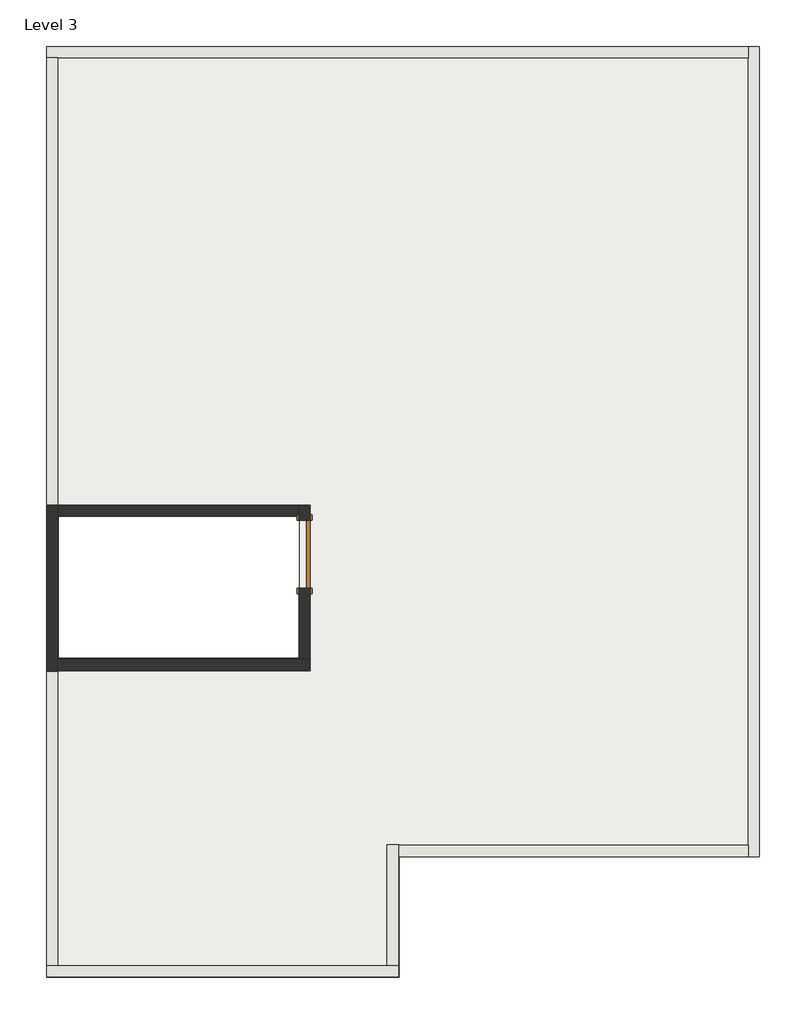
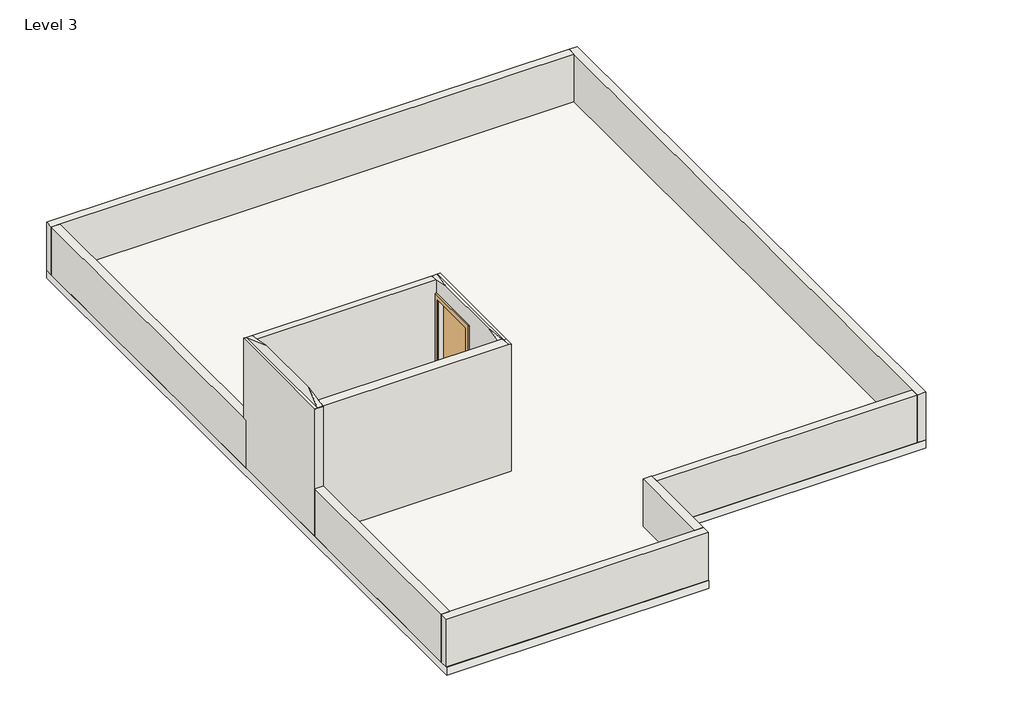
# One storey: 11 walls, 1 door, 1 slab.
"""IFC4 building model written with IfcOpenShell, lengths in millimetres."""

from ifc_helpers import new_model, si_unit, frame, origin, place, context, project, spatial, polyline, outline, extrude, faceted_brep, transform, mapped, element, save
from components import door_686f89d2

model = new_model("IFC4")

# Units and contexts
model_context = context("Model", 3, world=origin())
ifc_project = project(units=[si_unit("LENGTHUNIT", "METRE", prefix="MILLI")], contexts=[model_context])

# Site, building, storey
site = spatial("IfcSite", under=ifc_project)
building = spatial("IfcBuilding", under=site)
storey = spatial("IfcBuildingStorey", under=building, Name="Level 3", Elevation=6400.8)

# Door
placement = place(None, origin())
door_shape = door_686f89d2(model_context)
element("IfcDoor", 1, ObjectType="Single-Flush : 36\" x 84\"", at=placement, inside=storey, context=model_context, shape_type="MappedRepresentation", body=[
    mapped(door_shape, transform((-4237.5591614, 853.2825188, 6400.8), x_axis=(0.0, 1.0, 0.0), y_axis=(-1.0, 0.0, 0.0), z_axis=(0.0, 0.0, 1.0))),
])

# Slab
element("IfcSlab", 2, ObjectType="6\"", at=placement, inside=storey, context=model_context, shape_type="SweptSolid", body=[
    extrude(outline(polyline([(1887.7352982, 7685.8825188), (1887.7352982, -3216.5450563), (-2967.5591614, -3216.5450563), (-2967.5591614, -4842.6674812), (-7713.4647018, -4842.6674812), (-7713.4647018, 7685.8825188), (1887.7352982, 7685.8825188)]), holes=[polyline([(-4313.7591614, 1361.2825188), (-7548.3647018, 1361.2825188), (-7548.3647018, -543.1950563), (-4313.7591614, -543.1950563), (-4313.7591614, 1361.2825188)])]), frame((0.0, 0.0, 6248.4), z_axis=(0.0, 0.0, 1.0), x_axis=(1.0, 0.0, 0.0)), (0.0, 0.0, 1.0), 152.4),
])

# Walls
element("IfcWall", 3, ObjectType="6\"", at=placement, inside=storey, context=model_context, shape_type="Brep", body=[
    faceted_brep([(-7713.4647018, 7533.4825188, 6400.8), (-7561.0647018, 7533.4825188, 6400.8), (1735.3352982, 7533.4825188, 6400.8), (1735.3352982, 7533.4825188, 7315.2), (-7561.0647018, 7533.4825188, 7315.2), (-7713.4647018, 7533.4825188, 7315.2), (-7713.4647018, 7685.8825188, 6400.8), (-7713.4647018, 7685.8825188, 7315.2), (1735.3352982, 7685.8825188, 7315.2), (1735.3352982, 7685.8825188, 6400.8)], [[[0, 1, 2, 3, 4, 5]], [[6, 7, 8, 9]], [[2, 1, 0, 6, 9]], [[5, 4, 3, 8, 7]], [[0, 5, 7, 6]], [[3, 2, 9, 8]]]),
])
element("IfcWall", 4, ObjectType="6\"", at=placement, inside=storey, context=model_context, shape_type="SweptSolid", body=[
    extrude(outline(polyline([(-7561.0647018, -721.5174812), (-7561.0647018, -4683.9174812), (-7713.4647018, -4683.9174812), (-7713.4647018, -721.5174812), (-7561.0647018, -721.5174812)])), frame((0.0, 0.0, 6400.8), z_axis=(0.0, 0.0, 1.0), x_axis=(1.0, 0.0, 0.0)), (0.0, 0.0, 1.0), 914.4),
])
element("IfcWall", 5, ObjectType="6\"", at=placement, inside=storey, context=model_context, shape_type="Brep", body=[
    faceted_brep([(1735.3352982, 7685.8825188, 6400.8), (1735.3352982, 7533.4825188, 6400.8), (1735.3352982, -3064.1450563, 6400.8), (1735.3352982, -3216.5450563, 6400.8), (1735.3352982, -3216.5450563, 7315.2), (1735.3352982, -3064.1450563, 7315.2), (1735.3352982, 7533.4825188, 7315.2), (1735.3352982, 7685.8825188, 7315.2), (1887.7352982, 7685.8825188, 6400.8), (1887.7352982, 7685.8825188, 7315.2), (1887.7352982, -3216.5450563, 7315.2), (1887.7352982, -3216.5450563, 6400.8)], [[[0, 1, 2, 3, 4, 5, 6, 7]], [[8, 9, 10, 11]], [[3, 2, 1, 0, 8, 11]], [[7, 6, 5, 4, 10, 9]], [[0, 7, 9, 8]], [[4, 3, 11, 10]]]),
])
element("IfcWall", 6, ObjectType="6\"", at=placement, inside=storey, context=model_context, shape_type="SweptSolid", body=[
    extrude(outline(polyline([(1735.3352982, -3216.5450563), (-2976.3647018, -3216.5450563), (-2976.3647018, -3064.1450563), (1735.3352982, -3064.1450563), (1735.3352982, -3216.5450563)])), frame((0.0, 0.0, 6400.8), z_axis=(0.0, 0.0, 1.0), x_axis=(1.0, 0.0, 0.0)), (0.0, 0.0, 1.0), 914.4),
])
element("IfcWall", 7, ObjectType="6\"", at=placement, inside=storey, context=model_context, shape_type="Brep", body=[
    faceted_brep([(-4313.7591614, 1513.6825188, 6400.8), (-4313.7591614, 1361.2825188, 6400.8), (-4313.7591614, 1310.4825188, 6400.8), (-4313.7591614, 1310.4825188, 8534.4), (-4313.7591614, 396.0825188, 8534.4), (-4313.7591614, 396.0825188, 6400.8), (-4313.7591614, -562.2450563, 6400.8), (-4313.7591614, -562.2450563, 8865.7929338), (-4313.7591614, -264.7578497, 8917.7027606), (-4313.7591614, 1063.7953121, 8917.7027606), (-4313.7591614, 1361.2825188, 8865.7929338), (-4313.7591614, 1513.6825188, 8839.2), (-4161.3591614, 1310.4825188, 8534.4), (-4161.3591614, 1310.4825188, 6400.8), (-4161.3591614, 1513.6825188, 6400.8), (-4161.3591614, 1513.6825188, 8839.2), (-4161.3591614, -562.2450563, 8839.2), (-4161.3591614, -562.2450563, 6400.8), (-4161.3591614, 396.0825188, 6400.8), (-4161.3591614, 396.0825188, 8534.4), (-4209.088814, -562.2450563, 8839.2), (-4244.5460591, -562.2450563, 8865.7929338), (-4209.088814, 1513.6825188, 8839.2)], [[[0, 1, 2, 3, 4, 5, 6, 7, 8, 9, 10, 11]], [[12, 13, 14, 15, 16, 17, 18, 19]], [[18, 17, 6, 5]], [[14, 13, 2, 1, 0]], [[7, 6, 17, 16, 20, 21]], [[0, 11, 22, 15, 14]], [[11, 10, 9, 22]], [[9, 8, 21, 20, 22]], [[8, 7, 21]], [[20, 16, 15, 22]], [[3, 2, 13, 12]], [[4, 3, 12, 19]], [[5, 4, 19, 18]]]),
])
element("IfcWall", 8, ObjectType="6\"", at=placement, inside=storey, context=model_context, shape_type="Brep", body=[
    faceted_brep([(-4161.3591614, -562.2450563, 6400.8), (-4313.7591614, -562.2450563, 6400.8), (-7561.0647018, -562.2450563, 6400.8), (-7561.0647018, -562.2450563, 8865.7929338), (-4313.7591614, -562.2450563, 8865.7929338), (-4244.5460591, -562.2450563, 8865.7929338), (-4209.088814, -562.2450563, 8839.2), (-4161.3591614, -562.2450563, 8839.2), (-4161.3591614, -714.6450563, 6400.8), (-4161.3591614, -714.6450563, 8839.2), (-4209.088814, -714.6450563, 8839.2), (-7561.0647018, -714.6450563, 8839.2), (-7561.0647018, -714.6450563, 6400.8)], [[[0, 1, 2, 3, 4, 5, 6, 7]], [[8, 9, 10, 11, 12]], [[2, 1, 0, 8, 12]], [[0, 7, 9, 8]], [[3, 2, 12, 11]], [[5, 4, 3, 11, 10]], [[7, 6, 10, 9]], [[6, 5, 10]]]),
])
element("IfcWall", 9, ObjectType="6\"", at=placement, inside=storey, context=model_context, shape_type="Brep", body=[
    faceted_brep([(-7561.0647018, 1437.4825188, 6400.8), (-7561.0647018, 1513.6825188, 6400.8), (-7561.0647018, 7533.4825188, 6400.8), (-7561.0647018, 7533.4825188, 7315.2), (-7561.0647018, 1513.6825188, 7315.2), (-7561.0647018, 1437.4825188, 7315.2), (-7713.4647018, 1437.4825188, 6400.8), (-7713.4647018, 1437.4825188, 7315.2), (-7713.4647018, 1513.6825188, 7315.2), (-7713.4647018, 7533.4825188, 7315.2), (-7713.4647018, 7533.4825188, 6400.8)], [[[0, 1, 2, 3, 4, 5]], [[6, 7, 8, 9, 10]], [[2, 1, 0, 6, 10]], [[5, 4, 3, 9, 8, 7]], [[0, 5, 7, 6]], [[3, 2, 10, 9]]]),
])
element("IfcWall", 10, ObjectType="6\"", at=placement, inside=storey, context=model_context, shape_type="Brep", body=[
    faceted_brep([(-7561.0647018, -721.5174812, 6400.8), (-7561.0647018, -714.6450563, 6400.8), (-7561.0647018, -562.2450563, 6400.8), (-7561.0647018, 1361.2825188, 6400.8), (-7561.0647018, 1437.4825188, 6400.8), (-7561.0647018, 1437.4825188, 7315.2), (-7561.0647018, 1513.6825188, 7315.2), (-7561.0647018, 1513.6825188, 8839.2), (-7561.0647018, 1361.2825188, 8865.7929338), (-7561.0647018, 1063.7953121, 8917.7027606), (-7561.0647018, -264.7578497, 8917.7027606), (-7561.0647018, -562.2450563, 8865.7929338), (-7561.0647018, -714.6450563, 8839.2), (-7561.0647018, -721.5174812, 8839.2), (-7561.0647018, -721.5174812, 7315.2), (-7713.4647018, -721.5174812, 6400.8), (-7713.4647018, -721.5174812, 7315.2), (-7713.4647018, -721.5174812, 8839.2), (-7713.4647018, -714.6450563, 8839.2), (-7713.4647018, 1513.6825188, 8839.2), (-7713.4647018, 1513.6825188, 7315.2), (-7713.4647018, 1437.4825188, 7315.2), (-7713.4647018, 1437.4825188, 6400.8), (-7665.7350493, 1513.6825188, 8839.2), (-7665.7350493, -714.6450563, 8839.2)], [[[0, 1, 2, 3, 4, 5, 6, 7, 8, 9, 10, 11, 12, 13, 14]], [[15, 16, 17, 18, 19, 20, 21, 22]], [[4, 3, 2, 1, 0, 15, 22]], [[0, 14, 13, 17, 16, 15]], [[5, 4, 22, 21]], [[20, 6, 5, 21]], [[7, 6, 20, 19, 23]], [[13, 12, 24, 18, 17]], [[12, 11, 10, 24]], [[10, 9, 23, 24]], [[9, 8, 7, 23]], [[23, 19, 18, 24]]]),
])
element("IfcWall", 11, ObjectType="6\"", at=placement, inside=storey, context=model_context, shape_type="Brep", body=[
    faceted_brep([(-4313.7591614, 1513.6825188, 6400.8), (-7561.0647018, 1513.6825188, 6400.8), (-7561.0647018, 1513.6825188, 7315.2), (-7561.0647018, 1513.6825188, 8839.2), (-4313.7591614, 1513.6825188, 8839.2), (-4313.7591614, 1361.2825188, 6400.8), (-4313.7591614, 1361.2825188, 8865.7929338), (-7561.0647018, 1361.2825188, 8865.7929338), (-7561.0647018, 1361.2825188, 6400.8), (-7561.0647018, 1437.4825188, 6400.8)], [[[0, 1, 2, 3, 4]], [[5, 6, 7, 8]], [[1, 0, 5, 8, 9]], [[0, 4, 6, 5]], [[1, 9, 8, 7, 3, 2]], [[4, 3, 7, 6]]]),
])
element("IfcWall", 12, ObjectType="6\"", at=placement, inside=storey, context=model_context, shape_type="Brep", body=[
    faceted_brep([(-7713.4647018, -4836.3174812, 6400.8), (-2976.3647018, -4836.3174812, 6400.8), (-2976.3647018, -4836.3174812, 7315.2), (-7713.4647018, -4836.3174812, 7315.2), (-7713.4647018, -4683.9174812, 6400.8), (-7713.4647018, -4683.9174812, 7315.2), (-7561.0647018, -4683.9174812, 7315.2), (-3128.7647018, -4683.9174812, 7315.2), (-2976.3647018, -4683.9174812, 7315.2), (-2976.3647018, -4683.9174812, 6400.8), (-3128.7647018, -4683.9174812, 6400.8), (-7561.0647018, -4683.9174812, 6400.8)], [[[0, 1, 2, 3]], [[4, 5, 6, 7, 8, 9, 10, 11]], [[1, 0, 4, 11, 10, 9]], [[3, 2, 8, 7, 6, 5]], [[2, 1, 9, 8]], [[0, 3, 5, 4]]]),
])
element("IfcWall", 13, ObjectType="6\"", at=placement, inside=storey, context=model_context, shape_type="Brep", body=[
    faceted_brep([(-2976.3647018, -4683.9174812, 6400.8), (-2976.3647018, -3216.5450563, 6400.8), (-2976.3647018, -3064.1450563, 6400.8), (-2976.3647018, -3058.3174812, 6400.8), (-2976.3647018, -3058.3174812, 7315.2), (-2976.3647018, -3064.1450563, 7315.2), (-2976.3647018, -3216.5450563, 7315.2), (-2976.3647018, -4683.9174812, 7315.2), (-3128.7647018, -4683.9174812, 6400.8), (-3128.7647018, -4683.9174812, 7315.2), (-3128.7647018, -3058.3174812, 7315.2), (-3128.7647018, -3058.3174812, 6400.8)], [[[0, 1, 2, 3, 4, 5, 6, 7]], [[8, 9, 10, 11]], [[3, 2, 1, 0, 8, 11]], [[4, 3, 11, 10]], [[7, 6, 5, 4, 10, 9]], [[0, 7, 9, 8]]]),
])

save(model, "model.ifc")

# Revit data of these elements
# Type "Single-Flush : 36\" x 84\""
#   Type Mark = "1"
#   Construction Type Id = "MDOOR"
#   Assembly Code = "C1020"
#   Analytic Construction = "Metal"
#   Thickness = 0' - 2"
#   Heat Transfer Coefficient (U) = 0.651978 BTU/(h·ft²·°F)
#   Height = 7' - 0"
#   Trim Projection Ext = 0' - 1"
#   Trim Projection Int = 0' - 1"
#   Trim Width = 0' - 3"
#   Width = 3' - 0"
#   Define Thermal Properties by = 1
#   Door Material = Door - Panel
#   Frame Material = Door - Frame
#   Visual Light Transmittance = 0
#   Solar Heat Gain Coefficient = 0
#   Function = (empty or 0)
#   Wall Closure = (empty or 0)
# Type "6\""
#   Assembly Code = "B1010"
#   Function = 0
#   Layers, outside or top first: 0' - 6" "floor" (function 1)
# Type "6\""
#   Assembly Code = "B2010"
#   Layers, outside or top first: 0' - 6" "inner wall" (function 1)
# Element 1 (IfcDoor, "Single-Flush : 36\" x 84\"")
#   Phase Created = New Construction
#   Materials on its faces: "Door - Frame", "Door - Panel"
# Element 2 (IfcSlab, "6\"")
#   Height Offset From Level = 0' - 0"
#   Phase Created = New Construction
#   Materials on its faces: "floor"
# Elements 3, 4, 5, 6, 9, 12, 13 (IfcWall, "6\"")
#   Top Offset = 0' - 0"
#   Base Offset = 0' - 0"
#   Unconnected Height = 3' - 0"
#   wall height = 3' - 0"
#   Phase Created = New Construction
#   Base Constraint = Level 3
#   Materials on its faces: "inner wall"
# Elements 7, 8, 10, 11 (IfcWall, "6\"")
#   Top Offset = 0' - 0"
#   Base Offset = 0' - 0"
#   Unconnected Height = 8' - 0"
#   wall height = 8' - 0"
#   Phase Created = New Construction
#   Base Constraint = Level 3
#   Materials on its faces: "inner wall"
# Materials
#   "Door - Panel": class "Wood", colour RGB 210 159 95, transparency 0
#   "Door - Frame": colour RGB 118 70 51, transparency 0
#   "floor": class "Generic", colour RGB 128 100 74, transparency 0, Cost = 0
#   "inner wall": class "Generic", colour RGB 230 213 172, transparency 0, Cost = 0
